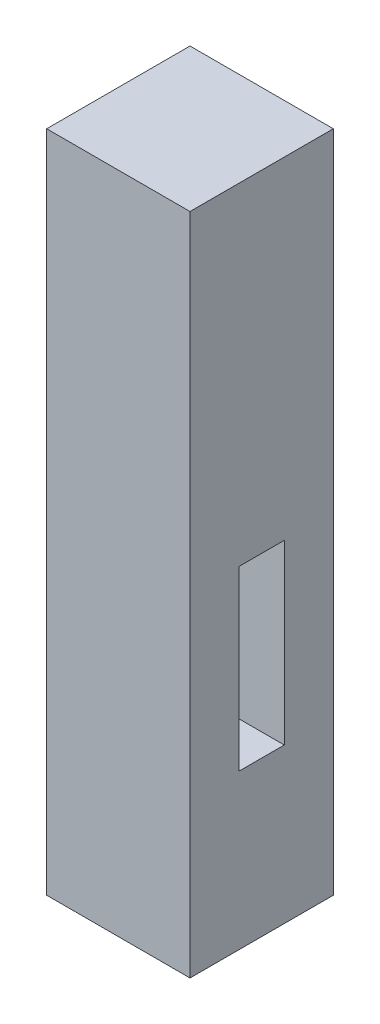
ISO-10303-21;
HEADER;
FILE_DESCRIPTION(('STEP AP214'),'2;1');
FILE_NAME('part.step','',(''),(''),'','','');
FILE_SCHEMA(('AUTOMOTIVE_DESIGN { 1 0 10303 214 1 1 1 1 }'));
ENDSEC;
DATA;
#1=APPLICATION_CONTEXT('core data for automotive mechanical design processes');
#2=APPLICATION_PROTOCOL_DEFINITION('international standard','automotive_design',2000,#1);
#3=PRODUCT_CONTEXT('',#1,'mechanical');
#4=PRODUCT('Part','Part','',(#3));
#5=PRODUCT_RELATED_PRODUCT_CATEGORY('part','',(#4));
#6=PRODUCT_DEFINITION_FORMATION('','',#4);
#7=PRODUCT_DEFINITION_CONTEXT('part definition',#1,'design');
#8=PRODUCT_DEFINITION('design','',#6,#7);
#9=PRODUCT_DEFINITION_SHAPE('','',#8);
#10=(LENGTH_UNIT() NAMED_UNIT(*) SI_UNIT(.MILLI.,.METRE.));
#11=(NAMED_UNIT(*) PLANE_ANGLE_UNIT() SI_UNIT($,.RADIAN.));
#12=(NAMED_UNIT(*) SI_UNIT($,.STERADIAN.) SOLID_ANGLE_UNIT());
#13=UNCERTAINTY_MEASURE_WITH_UNIT(LENGTH_MEASURE(1.E-05),#10,'distance_accuracy_value','');
#14=(GEOMETRIC_REPRESENTATION_CONTEXT(3) GLOBAL_UNCERTAINTY_ASSIGNED_CONTEXT((#13)) GLOBAL_UNIT_ASSIGNED_CONTEXT((#10,
#11,#12)) REPRESENTATION_CONTEXT('',''));
#15=CARTESIAN_POINT('',(0.,0.,0.));
#16=DIRECTION('',(0.,0.,1.));
#17=DIRECTION('',(1.,0.,0.));
#18=AXIS2_PLACEMENT_3D('',#15,#16,#17);
#19=CARTESIAN_POINT('',(19.,176.,19.));
#20=DIRECTION('',(-1.,0.,0.));
#21=DIRECTION('',(0.,0.,1.));
#22=AXIS2_PLACEMENT_3D('',#19,#20,#21);
#23=PLANE('',#22);
#24=DIRECTION('',(0.,0.,1.));
#25=VECTOR('',#24,1.);
#26=CARTESIAN_POINT('',(19.,88.,6.00000000000002));
#27=LINE('',#26,#25);
#28=CARTESIAN_POINT('',(19.,88.,-5.99999999999998));
#29=VERTEX_POINT('',#28);
#30=CARTESIAN_POINT('',(19.,88.,6.00000000000002));
#31=VERTEX_POINT('',#30);
#32=EDGE_CURVE('E113',#29,#31,#27,.T.);
#33=ORIENTED_EDGE('',*,*,#32,.F.);
#34=DIRECTION('',(0.,1.,0.));
#35=VECTOR('',#34,1.);
#36=CARTESIAN_POINT('',(19.,41.,-5.99999999999999));
#37=LINE('',#36,#35);
#38=CARTESIAN_POINT('',(19.,41.,-5.99999999999999));
#39=VERTEX_POINT('',#38);
#40=EDGE_CURVE('E52',#39,#29,#37,.T.);
#41=ORIENTED_EDGE('',*,*,#40,.F.);
#42=DIRECTION('',(0.,0.,-1.));
#43=VECTOR('',#42,1.);
#44=CARTESIAN_POINT('',(19.,41.,6.00000000000001));
#45=LINE('',#44,#43);
#46=CARTESIAN_POINT('',(19.,41.,6.00000000000001));
#47=VERTEX_POINT('',#46);
#48=EDGE_CURVE('E122',#47,#39,#45,.T.);
#49=ORIENTED_EDGE('',*,*,#48,.F.);
#50=DIRECTION('',(0.,-1.,0.));
#51=VECTOR('',#50,1.);
#52=CARTESIAN_POINT('',(19.,41.,6.00000000000001));
#53=LINE('',#52,#51);
#54=EDGE_CURVE('E106',#31,#47,#53,.T.);
#55=ORIENTED_EDGE('',*,*,#54,.F.);
#56=EDGE_LOOP('',(#33,#41,#49,#55));
#57=FACE_BOUND('',#56,.T.);
#58=DIRECTION('',(0.,0.,-1.));
#59=VECTOR('',#58,1.);
#60=CARTESIAN_POINT('',(19.,0.,19.));
#61=LINE('',#60,#59);
#62=CARTESIAN_POINT('',(19.,0.,19.));
#63=VERTEX_POINT('',#62);
#64=CARTESIAN_POINT('',(19.,0.,-19.));
#65=VERTEX_POINT('',#64);
#66=EDGE_CURVE('E126',#63,#65,#61,.T.);
#67=ORIENTED_EDGE('',*,*,#66,.T.);
#68=DIRECTION('',(0.,-1.,0.));
#69=VECTOR('',#68,1.);
#70=CARTESIAN_POINT('',(19.,176.,-19.));
#71=LINE('',#70,#69);
#72=CARTESIAN_POINT('',(19.,176.,-19.));
#73=VERTEX_POINT('',#72);
#74=EDGE_CURVE('E160',#73,#65,#71,.T.);
#75=ORIENTED_EDGE('',*,*,#74,.F.);
#76=DIRECTION('',(0.,0.,-1.));
#77=VECTOR('',#76,1.);
#78=CARTESIAN_POINT('',(19.,176.,19.));
#79=LINE('',#78,#77);
#80=CARTESIAN_POINT('',(19.,176.,19.));
#81=VERTEX_POINT('',#80);
#82=EDGE_CURVE('E132',#81,#73,#79,.T.);
#83=ORIENTED_EDGE('',*,*,#82,.F.);
#84=DIRECTION('',(0.,-1.,0.));
#85=VECTOR('',#84,1.);
#86=CARTESIAN_POINT('',(19.,176.,19.));
#87=LINE('',#86,#85);
#88=EDGE_CURVE('E143',#81,#63,#87,.T.);
#89=ORIENTED_EDGE('',*,*,#88,.T.);
#90=EDGE_LOOP('',(#67,#75,#83,#89));
#91=FACE_BOUND('',#90,.T.);
#92=ADVANCED_FACE('F39',(#57,#91),#23,.F.);
#93=CARTESIAN_POINT('',(-19.,176.,-19.));
#94=DIRECTION('',(0.,0.,1.));
#95=DIRECTION('',(1.,0.,0.));
#96=AXIS2_PLACEMENT_3D('',#93,#94,#95);
#97=PLANE('',#96);
#98=DIRECTION('',(-1.,0.,0.));
#99=VECTOR('',#98,1.);
#100=CARTESIAN_POINT('',(-19.,0.,-19.));
#101=LINE('',#100,#99);
#102=CARTESIAN_POINT('',(-19.,0.,-19.));
#103=VERTEX_POINT('',#102);
#104=EDGE_CURVE('E145',#65,#103,#101,.T.);
#105=ORIENTED_EDGE('',*,*,#104,.T.);
#106=DIRECTION('',(0.,-1.,0.));
#107=VECTOR('',#106,1.);
#108=CARTESIAN_POINT('',(-19.,176.,-19.));
#109=LINE('',#108,#107);
#110=CARTESIAN_POINT('',(-19.,176.,-19.));
#111=VERTEX_POINT('',#110);
#112=EDGE_CURVE('E152',#111,#103,#109,.T.);
#113=ORIENTED_EDGE('',*,*,#112,.F.);
#114=DIRECTION('',(-1.,0.,0.));
#115=VECTOR('',#114,1.);
#116=CARTESIAN_POINT('',(-19.,176.,-19.));
#117=LINE('',#116,#115);
#118=EDGE_CURVE('E131',#73,#111,#117,.T.);
#119=ORIENTED_EDGE('',*,*,#118,.F.);
#120=ORIENTED_EDGE('',*,*,#74,.T.);
#121=EDGE_LOOP('',(#105,#113,#119,#120));
#122=FACE_BOUND('',#121,.T.);
#123=ADVANCED_FACE('F183',(#122),#97,.F.);
#124=CARTESIAN_POINT('',(-19.,176.,19.));
#125=DIRECTION('',(1.,0.,0.));
#126=DIRECTION('',(0.,0.,-1.));
#127=AXIS2_PLACEMENT_3D('',#124,#125,#126);
#128=PLANE('',#127);
#129=DIRECTION('',(0.,0.,-1.));
#130=VECTOR('',#129,1.);
#131=CARTESIAN_POINT('',(-19.,41.,19.));
#132=LINE('',#131,#130);
#133=CARTESIAN_POINT('',(-19.,41.,6.00000000000001));
#134=VERTEX_POINT('',#133);
#135=CARTESIAN_POINT('',(-19.,41.,-5.99999999999999));
#136=VERTEX_POINT('',#135);
#137=EDGE_CURVE('E46',#134,#136,#132,.T.);
#138=ORIENTED_EDGE('',*,*,#137,.T.);
#139=DIRECTION('',(0.,1.,0.));
#140=VECTOR('',#139,1.);
#141=CARTESIAN_POINT('',(-19.,176.,-5.99999999999997));
#142=LINE('',#141,#140);
#143=CARTESIAN_POINT('',(-19.,88.,-5.99999999999998));
#144=VERTEX_POINT('',#143);
#145=EDGE_CURVE('E11',#136,#144,#142,.T.);
#146=ORIENTED_EDGE('',*,*,#145,.T.);
#147=DIRECTION('',(0.,0.,1.));
#148=VECTOR('',#147,1.);
#149=CARTESIAN_POINT('',(-19.,88.,19.));
#150=LINE('',#149,#148);
#151=CARTESIAN_POINT('',(-19.,88.,6.00000000000002));
#152=VERTEX_POINT('',#151);
#153=EDGE_CURVE('E159',#144,#152,#150,.T.);
#154=ORIENTED_EDGE('',*,*,#153,.T.);
#155=DIRECTION('',(0.,-1.,0.));
#156=VECTOR('',#155,1.);
#157=CARTESIAN_POINT('',(-19.,176.,6.00000000000003));
#158=LINE('',#157,#156);
#159=EDGE_CURVE('E108',#152,#134,#158,.T.);
#160=ORIENTED_EDGE('',*,*,#159,.T.);
#161=EDGE_LOOP('',(#138,#146,#154,#160));
#162=FACE_BOUND('',#161,.T.);
#163=DIRECTION('',(0.,0.,1.));
#164=VECTOR('',#163,1.);
#165=CARTESIAN_POINT('',(-19.,0.,19.));
#166=LINE('',#165,#164);
#167=CARTESIAN_POINT('',(-19.,0.,19.));
#168=VERTEX_POINT('',#167);
#169=EDGE_CURVE('E148',#103,#168,#166,.T.);
#170=ORIENTED_EDGE('',*,*,#169,.T.);
#171=DIRECTION('',(0.,-1.,0.));
#172=VECTOR('',#171,1.);
#173=CARTESIAN_POINT('',(-19.,176.,19.));
#174=LINE('',#173,#172);
#175=CARTESIAN_POINT('',(-19.,176.,19.));
#176=VERTEX_POINT('',#175);
#177=EDGE_CURVE('E151',#176,#168,#174,.T.);
#178=ORIENTED_EDGE('',*,*,#177,.F.);
#179=DIRECTION('',(0.,0.,1.));
#180=VECTOR('',#179,1.);
#181=CARTESIAN_POINT('',(-19.,176.,19.));
#182=LINE('',#181,#180);
#183=EDGE_CURVE('E140',#111,#176,#182,.T.);
#184=ORIENTED_EDGE('',*,*,#183,.F.);
#185=ORIENTED_EDGE('',*,*,#112,.T.);
#186=EDGE_LOOP('',(#170,#178,#184,#185));
#187=FACE_BOUND('',#186,.T.);
#188=ADVANCED_FACE('F163',(#162,#187),#128,.F.);
#189=CARTESIAN_POINT('',(-19.,176.,19.));
#190=DIRECTION('',(0.,0.,-1.));
#191=DIRECTION('',(-1.,0.,0.));
#192=AXIS2_PLACEMENT_3D('',#189,#190,#191);
#193=PLANE('',#192);
#194=DIRECTION('',(1.,0.,0.));
#195=VECTOR('',#194,1.);
#196=CARTESIAN_POINT('',(-19.,0.,19.));
#197=LINE('',#196,#195);
#198=EDGE_CURVE('E133',#168,#63,#197,.T.);
#199=ORIENTED_EDGE('',*,*,#198,.T.);
#200=ORIENTED_EDGE('',*,*,#88,.F.);
#201=DIRECTION('',(1.,0.,0.));
#202=VECTOR('',#201,1.);
#203=CARTESIAN_POINT('',(-19.,176.,19.));
#204=LINE('',#203,#202);
#205=EDGE_CURVE('E139',#176,#81,#204,.T.);
#206=ORIENTED_EDGE('',*,*,#205,.F.);
#207=ORIENTED_EDGE('',*,*,#177,.T.);
#208=EDGE_LOOP('',(#199,#200,#206,#207));
#209=FACE_BOUND('',#208,.T.);
#210=ADVANCED_FACE('F193',(#209),#193,.F.);
#211=CARTESIAN_POINT('',(0.,176.,0.));
#212=DIRECTION('',(0.,-1.,0.));
#213=DIRECTION('',(0.,0.,-1.));
#214=AXIS2_PLACEMENT_3D('',#211,#212,#213);
#215=PLANE('',#214);
#216=ORIENTED_EDGE('',*,*,#82,.T.);
#217=ORIENTED_EDGE('',*,*,#118,.T.);
#218=ORIENTED_EDGE('',*,*,#183,.T.);
#219=ORIENTED_EDGE('',*,*,#205,.T.);
#220=EDGE_LOOP('',(#216,#217,#218,#219));
#221=FACE_BOUND('',#220,.T.);
#222=ADVANCED_FACE('F179',(#221),#215,.F.);
#223=CARTESIAN_POINT('',(0.,0.,0.));
#224=DIRECTION('',(0.,-1.,0.));
#225=DIRECTION('',(0.,0.,-1.));
#226=AXIS2_PLACEMENT_3D('',#223,#224,#225);
#227=PLANE('',#226);
#228=ORIENTED_EDGE('',*,*,#66,.F.);
#229=ORIENTED_EDGE('',*,*,#198,.F.);
#230=ORIENTED_EDGE('',*,*,#169,.F.);
#231=ORIENTED_EDGE('',*,*,#104,.F.);
#232=EDGE_LOOP('',(#228,#229,#230,#231));
#233=FACE_BOUND('',#232,.T.);
#234=ADVANCED_FACE('F172',(#233),#227,.T.);
#235=CARTESIAN_POINT('',(-157.,41.,-5.99999999999999));
#236=DIRECTION('',(0.,0.,-1.));
#237=DIRECTION('',(0.,1.,0.));
#238=AXIS2_PLACEMENT_3D('',#235,#236,#237);
#239=PLANE('',#238);
#240=DIRECTION('',(1.,0.,0.));
#241=VECTOR('',#240,1.);
#242=CARTESIAN_POINT('',(-157.,41.,-5.99999999999999));
#243=LINE('',#242,#241);
#244=EDGE_CURVE('E127',#136,#39,#243,.T.);
#245=ORIENTED_EDGE('',*,*,#244,.T.);
#246=ORIENTED_EDGE('',*,*,#40,.T.);
#247=DIRECTION('',(1.,0.,0.));
#248=VECTOR('',#247,1.);
#249=CARTESIAN_POINT('',(-157.,88.,-5.99999999999998));
#250=LINE('',#249,#248);
#251=EDGE_CURVE('E115',#144,#29,#250,.T.);
#252=ORIENTED_EDGE('',*,*,#251,.F.);
#253=ORIENTED_EDGE('',*,*,#145,.F.);
#254=EDGE_LOOP('',(#245,#246,#252,#253));
#255=FACE_BOUND('',#254,.T.);
#256=ADVANCED_FACE('F166',(#255),#239,.F.);
#257=CARTESIAN_POINT('',(-157.,41.,6.00000000000001));
#258=DIRECTION('',(0.,-1.,0.));
#259=DIRECTION('',(0.,0.,-1.));
#260=AXIS2_PLACEMENT_3D('',#257,#258,#259);
#261=PLANE('',#260);
#262=DIRECTION('',(1.,0.,0.));
#263=VECTOR('',#262,1.);
#264=CARTESIAN_POINT('',(-157.,41.,6.00000000000001));
#265=LINE('',#264,#263);
#266=EDGE_CURVE('E112',#134,#47,#265,.T.);
#267=ORIENTED_EDGE('',*,*,#266,.T.);
#268=ORIENTED_EDGE('',*,*,#48,.T.);
#269=ORIENTED_EDGE('',*,*,#244,.F.);
#270=ORIENTED_EDGE('',*,*,#137,.F.);
#271=EDGE_LOOP('',(#267,#268,#269,#270));
#272=FACE_BOUND('',#271,.T.);
#273=ADVANCED_FACE('F169',(#272),#261,.F.);
#274=CARTESIAN_POINT('',(-157.,41.,6.00000000000001));
#275=DIRECTION('',(0.,0.,1.));
#276=DIRECTION('',(0.,-1.,0.));
#277=AXIS2_PLACEMENT_3D('',#274,#275,#276);
#278=PLANE('',#277);
#279=DIRECTION('',(1.,0.,0.));
#280=VECTOR('',#279,1.);
#281=CARTESIAN_POINT('',(-157.,88.,6.00000000000002));
#282=LINE('',#281,#280);
#283=EDGE_CURVE('E62',#152,#31,#282,.T.);
#284=ORIENTED_EDGE('',*,*,#283,.T.);
#285=ORIENTED_EDGE('',*,*,#54,.T.);
#286=ORIENTED_EDGE('',*,*,#266,.F.);
#287=ORIENTED_EDGE('',*,*,#159,.F.);
#288=EDGE_LOOP('',(#284,#285,#286,#287));
#289=FACE_BOUND('',#288,.T.);
#290=ADVANCED_FACE('F103',(#289),#278,.F.);
#291=CARTESIAN_POINT('',(-157.,88.,6.00000000000002));
#292=DIRECTION('',(0.,1.,0.));
#293=DIRECTION('',(0.,0.,1.));
#294=AXIS2_PLACEMENT_3D('',#291,#292,#293);
#295=PLANE('',#294);
#296=ORIENTED_EDGE('',*,*,#251,.T.);
#297=ORIENTED_EDGE('',*,*,#32,.T.);
#298=ORIENTED_EDGE('',*,*,#283,.F.);
#299=ORIENTED_EDGE('',*,*,#153,.F.);
#300=EDGE_LOOP('',(#296,#297,#298,#299));
#301=FACE_BOUND('',#300,.T.);
#302=ADVANCED_FACE('F117',(#301),#295,.F.);
#303=CLOSED_SHELL('',(#92,#123,#188,#210,#222,#234,#256,#273,#290,#302));
#304=MANIFOLD_SOLID_BREP('B2',#303);
#305=ADVANCED_BREP_SHAPE_REPRESENTATION('',(#18,#304),#14);
#306=SHAPE_DEFINITION_REPRESENTATION(#9,#305);
ENDSEC;
END-ISO-10303-21;
